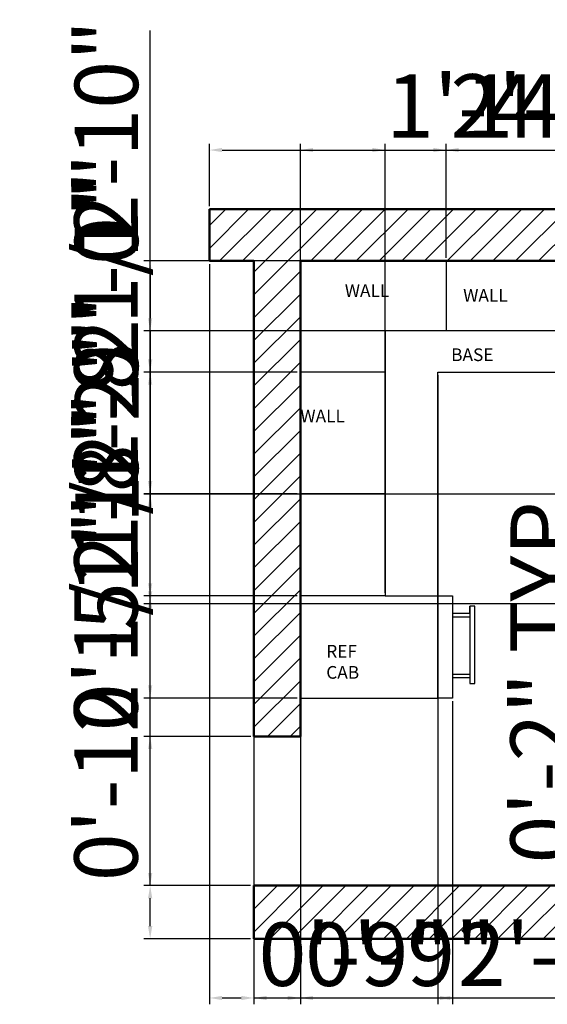
# Model space of a CAD drawing. Units: inches. Extents: x 1545 to 1898, y 1984 to 2198.
# Tile 1 of 4: x 1545 to 1649, y 2004 to 2198. Entities that reach past the tile are written whole.
import ezdxf

# ---------------------------------------------------------------- set-up
doc = ezdxf.new("R2010")
doc.units = ezdxf.units.IN
for name, color, linetype, lineweight in [('A-ANNO-DIMS', 2, 'Continuous', 18), ('A-ANNO-TEXT', 7, 'Continuous', 18), ('A-EQPM', 9, 'Continuous', 25), ('A-FLOR-CASE', 8, 'Continuous', 25), ('A-WALL', 7, 'Continuous', 50), ('A-WALL-PATT', 252, 'Continuous', 13)]:
    doc.layers.add(name, color=color, linetype=linetype, lineweight=lineweight)
doc.styles.get("Standard").update_dxf_attribs({"font": 'arial.ttf'})
doc.dimstyles.new('ISO-25', dxfattribs={"dimtxt": 12.5, "dimasz": 2.5, "dimexe": 1.25, "dimexo": 0.625, "dimtad": 1, "dimdec": 0, "dimlunit": 3, "dimtxsty": 'Standard', "dimcen": 2.5, "dimadec": 0, "dimazin": 0, "dimtfac": 1, "dimtdec": 0, "dimtmove": 0, "dimatfit": 3, "dimfxl": 1, "dimarcsym": 0})

# ---------------------------------------------------------------- blocks, each defined once
blk = doc.blocks.new('*D8')
at = {"layer": 'A-ANNO-DIMS', "color": 0, "lineweight": -2, "transparency": 16777216}
for p, q in [((1656.77, 2028.29), (1656.77, 2108.23)), ((1656.97, 2025.79), (1655.52, 2025.79)), ((1656.77, 2023.8), (1656.77, 2025.79)), ((1656.97, 2023.8), (1655.52, 2023.8)), ((1656.77, 2021.3), (1656.77, 2018.8))]:
    blk.add_line(p, q, dxfattribs=at)
at = {"layer": 'A-ANNO-DIMS', "color": 0, "transparency": 16777216}
for points in [[(1656.35, 2028.29), (1657.19, 2028.29), (1656.77, 2025.79)], [(1656.35, 2021.3), (1657.19, 2021.3), (1656.77, 2023.8)]]:
    blk.add_solid(points, dxfattribs=at)
at = {"layer": 'Defpoints', "color": 0, "transparency": 16777216}
for p in [(1656.77, 2025.79), (1657.6, 2025.79), (1657.6, 2023.8)]:
    blk.add_point(p, dxfattribs=at)
at = {"layer": 'A-ANNO-DIMS', "color": 0, "transparency": 16777216, "insert": (1649.76, 2069.51), "char_height": 12.5, "attachment_point": 5, "rotation": 90}
blk.add_mtext('0\'-2" TYP.', dxfattribs=at)
blk = doc.blocks.new('*D9')
at = {"layer": 'A-ANNO-DIMS', "color": 0, "lineweight": -2, "transparency": 16777216}
for p, q in [((1582.53, 2161.13), (1582.53, 2173.44)), ((1759.99, 2161.13), (1759.99, 2173.44)), ((1585.03, 2172.19), (1757.49, 2172.19))]:
    blk.add_line(p, q, dxfattribs=at)
at = {"layer": 'A-ANNO-DIMS', "color": 0, "transparency": 16777216}
for points in [[(1585.03, 2172.61), (1585.03, 2171.78), (1582.53, 2172.19)], [(1757.49, 2172.61), (1757.49, 2171.78), (1759.99, 2172.19)]]:
    blk.add_solid(points, dxfattribs=at)
at = {"layer": 'Defpoints', "color": 0, "transparency": 16777216}
for p in [(1759.99, 2172.19), (1582.53, 2160.51), (1759.99, 2160.51)]:
    blk.add_point(p, dxfattribs=at)
at = {"layer": 'A-ANNO-DIMS', "color": 0, "transparency": 16777216, "insert": (1671.26, 2179.28), "char_height": 12.5, "attachment_point": 5}
blk.add_mtext('14\'-9 1/2"', dxfattribs=at)
blk = doc.blocks.new('*D14')
at = {"layer": 'A-ANNO-DIMS', "color": 0, "lineweight": -2, "transparency": 16777216}
for p, q in [((1570.84, 2056.44), (1570.84, 2122.76)), ((1590.67, 2056.44), (1569.59, 2056.44)), ((1570.84, 2029.5), (1570.84, 2053.94)), ((1590.65, 2027), (1569.59, 2027))]:
    blk.add_line(p, q, dxfattribs=at)
at = {"layer": 'A-ANNO-DIMS', "color": 0, "transparency": 16777216}
for points in [[(1570.42, 2053.94), (1571.26, 2053.94), (1570.84, 2056.44)], [(1570.42, 2029.5), (1571.26, 2029.5), (1570.84, 2027)]]:
    blk.add_solid(points, dxfattribs=at)
at = {"layer": 'Defpoints', "color": 0, "transparency": 16777216}
for p in [(1570.84, 2056.44), (1591.3, 2056.44), (1591.27, 2027)]:
    blk.add_point(p, dxfattribs=at)
at = {"layer": 'A-ANNO-DIMS', "color": 0, "transparency": 16777216, "insert": (1563.75, 2090.85), "char_height": 12.5, "attachment_point": 5, "rotation": 90}
blk.add_mtext('2\'-5 1/2"', dxfattribs=at)
blk = doc.blocks.new('*D15')
at = {"layer": 'A-ANNO-DIMS', "color": 0, "lineweight": -2, "transparency": 16777216}
for p, q in [((1570.84, 2027), (1570.84, 2102.81)), ((1590.65, 2027), (1569.59, 2027)), ((1570.84, 2019.01), (1570.84, 2024.5)), ((1590.65, 2016.51), (1569.59, 2016.51))]:
    blk.add_line(p, q, dxfattribs=at)
at = {"layer": 'A-ANNO-DIMS', "color": 0, "transparency": 16777216}
for points in [[(1570.42, 2024.5), (1571.26, 2024.5), (1570.84, 2027)], [(1570.42, 2019.01), (1571.26, 2019.01), (1570.84, 2016.51)]]:
    blk.add_solid(points, dxfattribs=at)
at = {"layer": 'Defpoints', "color": 0, "transparency": 16777216}
for p in [(1570.84, 2027), (1591.27, 2027), (1591.27, 2016.51)]:
    blk.add_point(p, dxfattribs=at)
at = {"layer": 'A-ANNO-DIMS', "color": 0, "transparency": 16777216, "insert": (1563.75, 2066.15), "char_height": 12.5, "attachment_point": 5, "rotation": 90}
blk.add_mtext('0\'-10 1/2"', dxfattribs=at)
blk = doc.blocks.new('*D17')
at = {"layer": 'A-ANNO-DIMS', "color": 0, "lineweight": -2, "transparency": 16777216}
for p, q in [((1582.53, 2149.68), (1582.53, 2003.57)), ((1591.3, 2149.68), (1591.3, 2003.57)), ((1585.03, 2004.82), (1588.8, 2004.82)), ((1591.3, 2004.82), (1628.28, 2004.82))]:
    blk.add_line(p, q, dxfattribs=at)
at = {"layer": 'A-ANNO-DIMS', "color": 0, "transparency": 16777216}
for points in [[(1585.03, 2005.24), (1585.03, 2004.41), (1582.53, 2004.82)], [(1588.8, 2005.24), (1588.8, 2004.41), (1591.3, 2004.82)]]:
    blk.add_solid(points, dxfattribs=at)
at = {"layer": 'Defpoints', "color": 0, "transparency": 16777216}
for p in [(1582.53, 2150.3), (1591.3, 2150.3), (1591.3, 2004.82)]:
    blk.add_point(p, dxfattribs=at)
at = {"layer": 'A-ANNO-DIMS', "color": 0, "transparency": 16777216, "insert": (1611.04, 2011.83), "char_height": 12.5, "attachment_point": 5}
blk.add_mtext('0\'-9"', dxfattribs=at)
blk = doc.blocks.new('*D18')
at = {"layer": 'A-ANNO-DIMS', "color": 0, "lineweight": -2, "transparency": 16777216}
for p, q in [((1591.3, 2055.82), (1591.3, 2003.57)), ((1600.47, 2055.82), (1600.47, 2003.57)), ((1593.8, 2004.82), (1597.97, 2004.82)), ((1600.47, 2004.82), (1637.45, 2004.82))]:
    blk.add_line(p, q, dxfattribs=at)
at = {"layer": 'A-ANNO-DIMS', "color": 0, "transparency": 16777216}
for points in [[(1593.8, 2005.24), (1593.8, 2004.41), (1591.3, 2004.82)], [(1597.97, 2005.24), (1597.97, 2004.41), (1600.47, 2004.82)]]:
    blk.add_solid(points, dxfattribs=at)
at = {"layer": 'Defpoints', "color": 0, "transparency": 16777216}
for p in [(1591.3, 2056.44), (1600.47, 2056.44), (1600.47, 2004.82)]:
    blk.add_point(p, dxfattribs=at)
at = {"layer": 'A-ANNO-DIMS', "color": 0, "transparency": 16777216, "insert": (1620.21, 2011.83), "char_height": 12.5, "attachment_point": 5}
blk.add_mtext('0\'-9"', dxfattribs=at)
blk = doc.blocks.new('*D22')
at = {"layer": 'A-ANNO-DIMS', "color": 0, "lineweight": -2, "transparency": 16777216}
for p, q in [((1600.47, 2150.93), (1600.47, 2173.44)), ((1629.21, 2150.93), (1629.21, 2173.44)), ((1602.97, 2172.19), (1626.71, 2172.19)), ((1629.21, 2172.19), (1695.52, 2172.19))]:
    blk.add_line(p, q, dxfattribs=at)
at = {"layer": 'A-ANNO-DIMS', "color": 0, "transparency": 16777216}
for points in [[(1602.97, 2172.61), (1602.97, 2171.78), (1600.47, 2172.19)], [(1626.71, 2172.61), (1626.71, 2171.78), (1629.21, 2172.19)]]:
    blk.add_solid(points, dxfattribs=at)
at = {"layer": 'Defpoints', "color": 0, "transparency": 16777216}
for p in [(1629.21, 2172.19), (1600.47, 2150.3), (1629.21, 2150.3)]:
    blk.add_point(p, dxfattribs=at)
at = {"layer": 'A-ANNO-DIMS', "color": 0, "transparency": 16777216, "insert": (1663.61, 2179.28), "char_height": 12.5, "attachment_point": 5}
blk.add_mtext('2\'-4 1/2"', dxfattribs=at)
blk = doc.blocks.new('*D23')
at = {"layer": 'A-ANNO-DIMS', "color": 0, "lineweight": -2, "transparency": 16777216}
for p, q in [((1629.21, 2150.93), (1629.21, 2173.44)), ((1654.65, 2150.93), (1654.65, 2173.44)), ((1631.71, 2172.19), (1652.15, 2172.19)), ((1654.65, 2172.19), (1720.96, 2172.19))]:
    blk.add_line(p, q, dxfattribs=at)
at = {"layer": 'A-ANNO-DIMS', "color": 0, "transparency": 16777216}
for points in [[(1631.71, 2172.61), (1631.71, 2171.78), (1629.21, 2172.19)], [(1652.15, 2172.61), (1652.15, 2171.78), (1654.65, 2172.19)]]:
    blk.add_solid(points, dxfattribs=at)
at = {"layer": 'Defpoints', "color": 0, "transparency": 16777216}
for p in [(1654.65, 2172.19), (1629.21, 2150.3), (1654.65, 2150.3)]:
    blk.add_point(p, dxfattribs=at)
at = {"layer": 'A-ANNO-DIMS', "color": 0, "transparency": 16777216, "insert": (1689.05, 2179.28), "char_height": 12.5, "attachment_point": 5}
blk.add_mtext('2\'-1 1/2"', dxfattribs=at)
blk = doc.blocks.new('*D27')
at = {"layer": 'A-ANNO-DIMS', "color": 0, "lineweight": -2, "transparency": 16777216}
for p, q in [((1570.84, 2084.18), (1570.84, 2119.98)), ((1599.85, 2084.18), (1569.59, 2084.18)), ((1570.84, 2066.53), (1570.84, 2081.68)), ((1599.85, 2064.03), (1569.59, 2064.03))]:
    blk.add_line(p, q, dxfattribs=at)
at = {"layer": 'A-ANNO-DIMS', "color": 0, "transparency": 16777216}
for points in [[(1570.42, 2081.68), (1571.26, 2081.68), (1570.84, 2084.18)], [(1570.42, 2066.53), (1571.26, 2066.53), (1570.84, 2064.03)]]:
    blk.add_solid(points, dxfattribs=at)
at = {"layer": 'Defpoints', "color": 0, "transparency": 16777216}
for p in [(1570.84, 2084.18), (1600.47, 2084.18), (1600.47, 2064.03)]:
    blk.add_point(p, dxfattribs=at)
at = {"layer": 'A-ANNO-DIMS', "color": 0, "transparency": 16777216, "insert": (1563.83, 2103.33), "char_height": 12.5, "attachment_point": 5, "rotation": 90}
blk.add_mtext('1\'-8"', dxfattribs=at)
blk = doc.blocks.new('*D28')
at = {"layer": 'A-ANNO-DIMS', "color": 0, "lineweight": -2, "transparency": 16777216}
for p, q in [((1570.84, 2104.34), (1570.84, 2140.14)), ((1599.85, 2104.34), (1569.59, 2104.34)), ((1570.84, 2086.68), (1570.84, 2101.84)), ((1599.85, 2084.18), (1569.59, 2084.18))]:
    blk.add_line(p, q, dxfattribs=at)
at = {"layer": 'A-ANNO-DIMS', "color": 0, "transparency": 16777216}
for points in [[(1570.42, 2101.84), (1571.26, 2101.84), (1570.84, 2104.34)], [(1570.42, 2086.68), (1571.26, 2086.68), (1570.84, 2084.18)]]:
    blk.add_solid(points, dxfattribs=at)
at = {"layer": 'Defpoints', "color": 0, "transparency": 16777216}
for p in [(1570.84, 2104.34), (1600.47, 2104.34), (1600.47, 2084.18)]:
    blk.add_point(p, dxfattribs=at)
at = {"layer": 'A-ANNO-DIMS', "color": 0, "transparency": 16777216, "insert": (1563.83, 2123.49), "char_height": 12.5, "attachment_point": 5, "rotation": 90}
blk.add_mtext('1\'-8"', dxfattribs=at)
blk = doc.blocks.new('*D29')
at = {"layer": 'A-ANNO-DIMS', "color": 0, "lineweight": -2, "transparency": 16777216}
for p, q in [((1570.84, 2128.36), (1570.84, 2165.55)), ((1599.85, 2128.36), (1569.59, 2128.36)), ((1570.84, 2106.84), (1570.84, 2125.86)), ((1599.85, 2104.34), (1569.59, 2104.34))]:
    blk.add_line(p, q, dxfattribs=at)
at = {"layer": 'A-ANNO-DIMS', "color": 0, "transparency": 16777216}
for points in [[(1570.42, 2125.86), (1571.26, 2125.86), (1570.84, 2128.36)], [(1570.42, 2106.84), (1571.26, 2106.84), (1570.84, 2104.34)]]:
    blk.add_solid(points, dxfattribs=at)
at = {"layer": 'Defpoints', "color": 0, "transparency": 16777216}
for p in [(1570.84, 2128.36), (1600.47, 2128.36), (1600.47, 2104.34)]:
    blk.add_point(p, dxfattribs=at)
at = {"layer": 'A-ANNO-DIMS', "color": 0, "transparency": 16777216, "insert": (1563.83, 2148.21), "char_height": 12.5, "attachment_point": 5, "rotation": 90}
blk.add_mtext('2\'-0"', dxfattribs=at)
blk = doc.blocks.new('*D30')
at = {"layer": 'A-ANNO-DIMS', "color": 0, "lineweight": -2, "transparency": 16777216}
for p, q in [((1570.84, 2150.3), (1570.84, 2195.82)), ((1599.85, 2150.3), (1569.59, 2150.3)), ((1570.84, 2130.86), (1570.84, 2147.8)), ((1599.85, 2128.36), (1569.59, 2128.36))]:
    blk.add_line(p, q, dxfattribs=at)
at = {"layer": 'A-ANNO-DIMS', "color": 0, "transparency": 16777216}
for points in [[(1570.42, 2147.8), (1571.26, 2147.8), (1570.84, 2150.3)], [(1570.42, 2130.86), (1571.26, 2130.86), (1570.84, 2128.36)]]:
    blk.add_solid(points, dxfattribs=at)
at = {"layer": 'Defpoints', "color": 0, "transparency": 16777216}
for p in [(1570.84, 2150.3), (1600.47, 2150.3), (1600.47, 2128.36)]:
    blk.add_point(p, dxfattribs=at)
at = {"layer": 'A-ANNO-DIMS', "color": 0, "transparency": 16777216, "insert": (1563.83, 2174.31), "char_height": 12.5, "attachment_point": 5, "rotation": 90}
blk.add_mtext('1\'-10"', dxfattribs=at)
blk = doc.blocks.new('*D34')
at = {"layer": 'A-ANNO-DIMS', "color": 0, "lineweight": -2, "transparency": 16777216}
for p, q in [((1570.84, 2104.25), (1570.84, 2169.18)), ((1732.77, 2104.25), (1569.59, 2104.25)), ((1570.84, 2085.11), (1570.84, 2101.75)), ((1732.77, 2082.61), (1569.59, 2082.61))]:
    blk.add_line(p, q, dxfattribs=at)
at = {"layer": 'A-ANNO-DIMS', "color": 0, "transparency": 16777216}
for points in [[(1570.42, 2101.75), (1571.26, 2101.75), (1570.84, 2104.25)], [(1570.42, 2085.11), (1571.26, 2085.11), (1570.84, 2082.61)]]:
    blk.add_solid(points, dxfattribs=at)
at = {"layer": 'Defpoints', "color": 0, "transparency": 16777216}
for p in [(1570.84, 2104.25), (1733.39, 2104.25), (1733.39, 2082.61)]:
    blk.add_point(p, dxfattribs=at)
at = {"layer": 'A-ANNO-DIMS', "color": 0, "transparency": 16777216, "insert": (1563.75, 2137.96), "char_height": 12.5, "attachment_point": 5, "rotation": 90}
blk.add_mtext('1\'-9 1/2"', dxfattribs=at)
blk = doc.blocks.new('*D36')
at = {"layer": 'A-ANNO-DIMS', "color": 0, "lineweight": -2, "transparency": 16777216}
for p, q in [((1600.47, 2063.41), (1600.47, 2003.57)), ((1630.49, 2063.41), (1630.49, 2003.57)), ((1602.97, 2004.82), (1627.99, 2004.82)), ((1630.49, 2004.82), (1667.68, 2004.82))]:
    blk.add_line(p, q, dxfattribs=at)
at = {"layer": 'A-ANNO-DIMS', "color": 0, "transparency": 16777216}
for points in [[(1602.97, 2005.24), (1602.97, 2004.41), (1600.47, 2004.82)], [(1627.99, 2005.24), (1627.99, 2004.41), (1630.49, 2004.82)]]:
    blk.add_solid(points, dxfattribs=at)
at = {"layer": 'Defpoints', "color": 0, "transparency": 16777216}
for p in [(1600.47, 2064.03), (1630.49, 2064.03), (1630.49, 2004.82)]:
    blk.add_point(p, dxfattribs=at)
at = {"layer": 'A-ANNO-DIMS', "color": 0, "transparency": 16777216, "insert": (1650.33, 2011.83), "char_height": 12.5, "attachment_point": 5}
blk.add_mtext('2\'-6"', dxfattribs=at)
blk = doc.blocks.new('*D38')
at = {"layer": 'A-ANNO-DIMS', "color": 0, "lineweight": -2, "transparency": 16777216}
for p, q in [((1627.57, 2127.73), (1627.57, 2003.57)), ((1733.39, 2122.03), (1733.39, 2003.57)), ((1630.07, 2004.82), (1730.89, 2004.82))]:
    blk.add_line(p, q, dxfattribs=at)
at = {"layer": 'A-ANNO-DIMS', "color": 0, "transparency": 16777216}
for points in [[(1630.07, 2005.24), (1630.07, 2004.41), (1627.57, 2004.82)], [(1730.89, 2005.24), (1730.89, 2004.41), (1733.39, 2004.82)]]:
    blk.add_solid(points, dxfattribs=at)
at = {"layer": 'Defpoints', "color": 0, "transparency": 16777216}
for p in [(1627.57, 2128.35), (1733.39, 2122.65), (1733.39, 2004.82)]:
    blk.add_point(p, dxfattribs=at)
at = {"layer": 'A-ANNO-DIMS', "color": 0, "transparency": 16777216, "insert": (1680.48, 2011.83), "char_height": 12.5, "attachment_point": 5}
blk.add_mtext('8\'-10"', dxfattribs=at)
blk = doc.blocks.new('*D39')
at = {"layer": 'A-ANNO-DIMS', "color": 0, "lineweight": -2, "transparency": 16777216}
for p, q in [((1628.58, 2150.3), (1569.59, 2150.3)), ((1570.84, 2147.8), (1570.84, 2138.98)), ((1628.58, 2136.48), (1569.59, 2136.48)), ((1570.84, 2136.48), (1570.84, 2100.68))]:
    blk.add_line(p, q, dxfattribs=at)
at = {"layer": 'A-ANNO-DIMS', "color": 0, "transparency": 16777216}
for points in [[(1570.42, 2147.8), (1571.26, 2147.8), (1570.84, 2150.3)], [(1570.42, 2138.98), (1571.26, 2138.98), (1570.84, 2136.48)]]:
    blk.add_solid(points, dxfattribs=at)
at = {"layer": 'Defpoints', "color": 0, "transparency": 16777216}
for p in [(1629.21, 2150.3), (1570.84, 2136.48), (1629.21, 2136.48)]:
    blk.add_point(p, dxfattribs=at)
at = {"layer": 'A-ANNO-DIMS', "color": 0, "transparency": 16777216, "insert": (1563.94, 2117.33), "char_height": 12.5, "attachment_point": 5, "rotation": 90}
blk.add_mtext('1\'-2"', dxfattribs=at)
blk = doc.blocks.new('*D40')
at = {"layer": 'A-ANNO-DIMS', "color": 0, "lineweight": -2, "transparency": 16777216}
for p, q in [((1600.47, 2084.8), (1600.47, 2173.44)), ((1617.18, 2084.8), (1617.18, 2173.44)), ((1602.97, 2172.19), (1614.68, 2172.19)), ((1617.18, 2172.19), (1682.11, 2172.19))]:
    blk.add_line(p, q, dxfattribs=at)
at = {"layer": 'A-ANNO-DIMS', "color": 0, "transparency": 16777216}
for points in [[(1602.97, 2172.61), (1602.97, 2171.78), (1600.47, 2172.19)], [(1614.68, 2172.61), (1614.68, 2171.78), (1617.18, 2172.19)]]:
    blk.add_solid(points, dxfattribs=at)
at = {"layer": 'Defpoints', "color": 0, "transparency": 16777216}
for p in [(1617.18, 2172.19), (1600.47, 2084.18), (1617.18, 2084.18)]:
    blk.add_point(p, dxfattribs=at)
at = {"layer": 'A-ANNO-DIMS', "color": 0, "transparency": 16777216, "insert": (1650.89, 2179.28), "char_height": 12.5, "attachment_point": 5}
blk.add_mtext('1\'-4 1/2"', dxfattribs=at)

msp = doc.modelspace()

# ---------------------------------------------------------------- hatches: boundary and pattern name
at = {"layer": 'A-WALL-PATT'}
h = msp.add_hatch(dxfattribs=at)
h.set_pattern_fill('ANSI31', color=256)
h.paths.add_polyline_path([(1759.99, 2160.51), (1639.99, 2160.51), (1582.53, 2160.51), (1582.53, 2150.3), (1591.3, 2150.3), (1591.3, 2056.44), (1600.47, 2056.44), (1600.47, 2150.3), (1751.61, 2150.3), (1751.61, 2119.93), (1759.99, 2119.93)])
h.paths.add_polyline_path([(1759.99, 2079.5), (1751.61, 2079.5), (1751.61, 2057.94), (1759.99, 2057.94)], flags=17)
h.paths.add_polyline_path([(1599.8, 2117.08), (1610.56, 2117.08), (1610.56, 2122.23), (1599.8, 2122.23)], flags=24)
h = msp.add_hatch(dxfattribs=at)
h.set_pattern_fill('ANSI31', color=256)
h.paths.add_polyline_path([(1656.39, 2027), (1591.27, 2027), (1591.27, 2016.51), (1604.23, 2016.51), (1656.39, 2016.51)])
h.paths.add_polyline_path([(1759.99, 2034.9), (1751.61, 2034.9), (1751.61, 2027), (1697.47, 2027), (1697.47, 2016.51), (1759.99, 2016.51)])

# ---------------------------------------------------------------- linework, layer by layer
at = {"layer": 'A-EQPM'}
for p, q in [((1600.47, 2084.18), (1600.47, 2064.03)), ((1627.57, 2064.03), (1627.57, 2084.18)), ((1627.57, 2084.18), (1630.49, 2084.18)), ((1630.49, 2084.18), (1630.49, 2064.03)), ((1633.89, 2080.8), (1633.89, 2082.16)), ((1633.89, 2082.16), (1633.89, 2066.9)), ((1634.85, 2082.16), (1633.89, 2082.16)), ((1634.85, 2066.9), (1634.85, 2082.16)), ((1630.49, 2080.8), (1633.89, 2080.8)), ((1633.89, 2080), (1630.49, 2080)), ((1630.49, 2080), (1630.49, 2068.77)), ((1633.89, 2080.8), (1633.89, 2080)), ((1630.49, 2068.77), (1633.89, 2068.77)), ((1633.89, 2068.02), (1630.49, 2068.02)), ((1633.89, 2068.77), (1633.89, 2068.02)), ((1633.89, 2066.9), (1634.85, 2066.9)), ((1600.47, 2064.03), (1627.57, 2064.03)), ((1630.49, 2064.03), (1627.57, 2064.03))]:
    msp.add_line(p, q, dxfattribs=at)
at = {"layer": 'A-FLOR-CASE'}
for p, q in [((1629.21, 2150.3), (1629.21, 2136.48)), ((1654.65, 2136.48), (1617.18, 2136.48)), ((1617.18, 2136.48), (1617.18, 2084.18)), ((1617.18, 2128.36), (1600.47, 2128.36)), ((1627.57, 2084.18), (1627.57, 2128.35)), ((1627.57, 2128.35), (1654.65, 2128.35)), ((1617.18, 2104.34), (1600.47, 2104.34)), ((1617.18, 2084.18), (1600.47, 2084.18)), ((1617.18, 2084.18), (1627.57, 2084.18))]:
    msp.add_line(p, q, dxfattribs=at)
at = {"layer": 'A-WALL'}
for p, q in [((1582.53, 2160.51), (1639.99, 2160.51)), ((1582.53, 2160.51), (1582.53, 2150.3)), ((1639.99, 2160.51), (1759.99, 2160.51)), ((1582.53, 2150.3), (1591.3, 2150.3)), ((1591.3, 2056.44), (1591.3, 2150.3)), ((1600.47, 2150.3), (1600.47, 2056.44)), ((1600.47, 2150.3), (1751.61, 2150.3)), ((1600.47, 2056.44), (1591.3, 2056.44)), ((1591.27, 2027), (1591.27, 2016.51)), ((1656.39, 2027), (1591.27, 2027)), ((1591.27, 2016.51), (1604.23, 2016.51)), ((1656.39, 2016.51), (1604.23, 2016.51))]:
    msp.add_line(p, q, dxfattribs=at)

# ---------------------------------------------------------------- texts
at = {"layer": 'A-ANNO-TEXT', "char_height": 2.5, "attachment_point": 1}
for s, width, insert in [('WALL', 19.5596, (1609.23, 2145.69)), ('WALL', 15.901, (1632.58, 2144.74)), ('BASE', 14.4938, (1630.2, 2133.04)), ('WALL', 16.7076, (1600.47, 2120.94)), ('REF\\PCAB', 18.1524, (1605.57, 2074.51))]:
    msp.add_mtext_dynamic_manual_height_columns(s, width=width, gutter_width=12.5, heights=[0], dxfattribs=dict(at, insert=insert))

# ---------------------------------------------------------------- dimensions: what is measured, and where the dimension line sits
at = {"layer": 'A-ANNO-DIMS'}
for base, p1, p2, picture, middle in [((1570.84, 2150.3), (1600.47, 2128.36), (1600.47, 2150.3), '*D30', (1563.83, 2174.31)), ((1570.84, 2104.25), (1733.39, 2082.61), (1733.39, 2104.25), '*D34', (1563.75, 2137.96)), ((1570.84, 2128.36), (1600.47, 2104.34), (1600.47, 2128.36), '*D29', (1563.83, 2148.21)), ((1570.84, 2136.48), (1629.21, 2150.3), (1629.21, 2136.48), '*D39', (1563.94, 2117.33)), ((1570.84, 2104.34), (1600.47, 2084.18), (1600.47, 2104.34), '*D28', (1563.83, 2123.49)), ((1570.84, 2056.44), (1591.27, 2027), (1591.3, 2056.44), '*D14', (1563.75, 2090.85)), ((1570.8401, 2084.176), (1600.4713, 2064.0329), (1600.4713, 2084.176), '*D27', (1563.833, 2103.3268)), ((1570.84, 2027), (1591.27, 2016.51), (1591.27, 2027), '*D15', (1563.75, 2066.15))]:
    dim = msp.add_linear_dim(base=base, p1=p1, p2=p2, angle=90, dimstyle='ISO-25', override={"dimdec": 1, "dimlfac": 1, "dimrnd": 0, "dimzin": 1, "dimdsep": 46, "dimlunit": 4, "dimfrac": 2}, dxfattribs=at)
    dim.commit()
    dim.dimension.update_dxf_attribs({"geometry": picture, "text_midpoint": middle})
for base, p1, p2, picture, middle in [((1759.99, 2172.19), (1582.53, 2160.51), (1759.99, 2160.51), '*D9', (1671.26, 2179.28)), ((1629.21, 2172.19), (1600.47, 2150.3), (1629.21, 2150.3), '*D22', (1663.61, 2179.28)), ((1617.18, 2172.19), (1600.47, 2084.18), (1617.18, 2084.18), '*D40', (1650.89, 2179.28)), ((1654.65, 2172.19), (1629.21, 2150.3), (1654.65, 2150.3), '*D23', (1689.05, 2179.28)), ((1591.3, 2004.82), (1582.53, 2150.3), (1591.3, 2150.3), '*D17', (1611.04, 2011.83)), ((1733.39, 2004.82), (1627.57, 2128.35), (1733.39, 2122.65), '*D38', (1680.48, 2011.83)), ((1630.49, 2004.82), (1600.47, 2064.03), (1630.49, 2064.03), '*D36', (1650.33, 2011.83)), ((1600.47, 2004.82), (1591.3, 2056.44), (1600.47, 2056.44), '*D18', (1620.21, 2011.83))]:
    dim = msp.add_linear_dim(base=base, p1=p1, p2=p2, dimstyle='ISO-25', override={"dimdec": 1, "dimlfac": 1, "dimrnd": 0, "dimzin": 1, "dimdsep": 46, "dimlunit": 4, "dimfrac": 2}, dxfattribs=at)
    dim.commit()
    dim.dimension.update_dxf_attribs({"geometry": picture, "text_midpoint": middle})
dim = msp.add_linear_dim(base=(1656.77, 2025.79), p1=(1657.6, 2023.8), p2=(1657.6, 2025.79), angle=90, text='<> TYP.', dimstyle='ISO-25', override={"dimdec": 1, "dimlfac": 1, "dimrnd": 0, "dimzin": 1, "dimdsep": 46, "dimlunit": 4, "dimfrac": 2}, dxfattribs=at)
dim.commit()
dim.dimension.update_dxf_attribs({"geometry": '*D8', "text_midpoint": (1649.76, 2069.51)})

doc.saveas('drawing.dxf')
